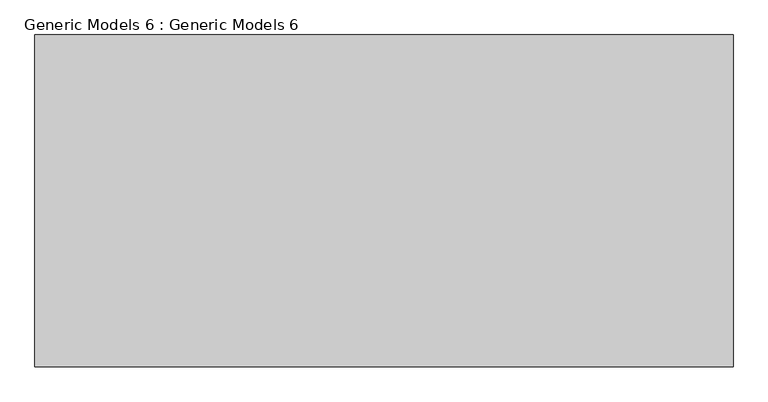
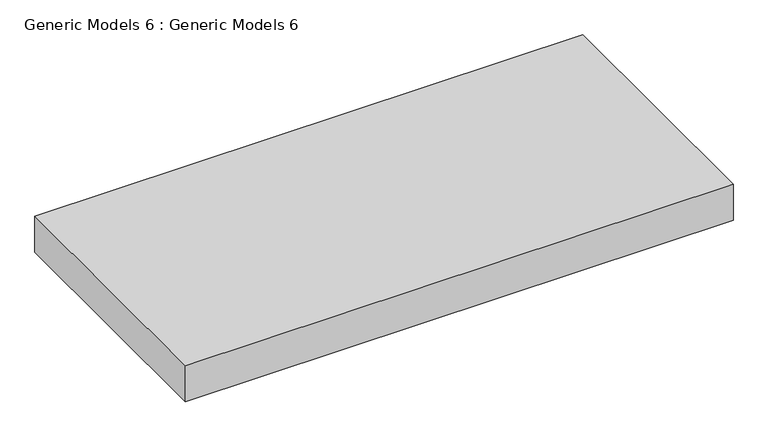
"""IFC4 building model written with IfcOpenShell, lengths in millimetres: proxy geometry, Generic Models 6 : Generic Models 6."""

from ifc_helpers import new_model, si_unit, frame, origin, place, context, project, spatial, polyline, outline, extrude, source, transform, mapped, element, save


def generic_models_6_generic_models_6_4fc6bb2b(model_context):
    return source(origin(), model_context, "Body", "SweptSolid", [
        extrude(outline(polyline([(-10521.0371373, -3685.061407), (-14902.5371373, -3685.061407), (-14902.5371373, -1602.261407), (-10521.0371373, -1602.261407), (-10521.0371373, -3685.061407)])), frame((0.0, 0.0, 6121.4), z_axis=(0.0, 0.0, 1.0), x_axis=(1.0, 0.0, 0.0)), (0.0, 0.0, 1.0), 304.8),
    ])


if __name__ == "__main__":
    model = new_model("IFC4")
    model_context = context("Model", 3, world=origin())
    ifc_project = project(units=[si_unit("LENGTHUNIT", "METRE", prefix="MILLI")], contexts=[model_context])
    site = spatial("IfcSite", under=ifc_project)
    building = spatial("IfcBuilding", under=site)
    placement = place(None, origin())
    generic_models_6_generic_models_6_shape = generic_models_6_generic_models_6_4fc6bb2b(model_context)
    element("IfcBuildingElementProxy", 1, Name="Generic Models 6 : Generic Models 6", ObjectType="Generic Models 6 : Generic Models 6", at=placement, inside=building, context=model_context, shape_type="MappedRepresentation", body=[
        mapped(generic_models_6_generic_models_6_shape, transform((0.0, 0.0, 0.0), x_axis=(1.0, 0.0, 0.0), y_axis=(0.0, 1.0, 0.0), z_axis=(0.0, 0.0, 1.0))),
    ])
    save(model, "model.ifc")

# Revit data of these elements
# Element 1 (IfcBuildingElementProxy, "Generic Models 6 : Generic Models 6")
#   Materials on its faces: "Gypsum Wall Board"
# Materials
#   "Gypsum Wall Board": class "Generic", colour RGB 127 127 127, transparency 0, Description = "Gypsum Wall Board", Cost = 0
